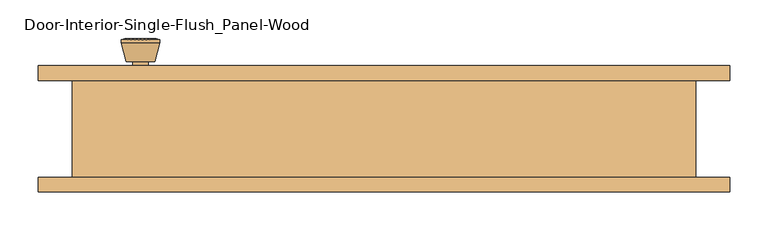
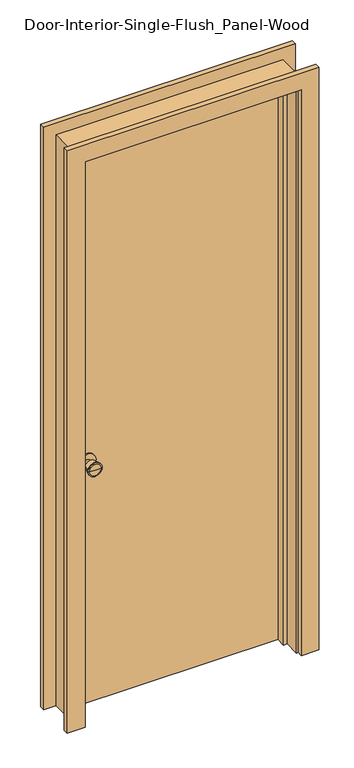
"""IFC4 building model written with IfcOpenShell, lengths in millimetres: door geometry, Door-Interior-Single-Flush_Panel-Wood."""

from ifc_helpers import new_model, si_unit, point, frame, frame_2d, origin, origin_with_axes, place, context, project, spatial, polyline, circle_curve, trimmed, segment, composite_curve, outline, extrude, faceted_brep, source, transform, mapped, element, save
from ifc_brep_helpers import plane_surface, cylinder_surface, revolved_surface, advanced_brep


def door_interior_single_flush_panel_wood_df77f4d3(model_context):
    return source(origin(), model_context, "Body", "SolidModel", [
        advanced_brep(
        [(-317.5, 19.4, 914.4), (-307.5, 19.4, 914.4), (-327.5, 19.4, 914.4), (-297.0241324, -29.6, 914.4), (-317.5, -29.6, 914.4), (-337.9758676, -29.6, 914.4), (-292.5, -27.7721319, 914.4), (-342.5, -27.7721319, 914.4), (-292.5, -24.3084537, 914.4), (-342.5, -24.3084537, 914.4), (-298.863764, 0.4, 914.4), (-336.136236, 0.4, 914.4), (-307.5, 0.4, 914.4), (-327.5, 0.4, 914.4)],
        [
            (0, 1),
            (1, 2, circle_curve(frame((-317.5, 19.4, 914.4), z_axis=(0.0, 1.0, 0.0), x_axis=(-1.0, 0.0, 0.0)), 10.0)),
            (2, 0),
            (2, 1, circle_curve(frame((-317.5, 19.4, 914.4), z_axis=(0.0, 1.0, 0.0), x_axis=(-1.0, 0.0, 0.0)), 10.0)),
            (3, 4),
            (4, 5),
            (5, 3, circle_curve(frame((-317.5, -29.6, 914.4), z_axis=(0.0, -1.0, 0.0), x_axis=(-1.0, 0.0, 0.0)), 20.4758676)),
            (3, 5, circle_curve(frame((-317.5, -29.6, 914.4), z_axis=(0.0, -1.0, 0.0), x_axis=(-1.0, 0.0, 0.0)), 20.4758676)),
            (6, 3),
            (5, 7),
            (7, 6, circle_curve(frame((-317.5, -27.7721319, 914.4), z_axis=(0.0, -1.0, 0.0), x_axis=(-1.0, 0.0, 0.0)), 25.0)),
            (6, 7, circle_curve(frame((-317.5, -27.7721319, 914.4), z_axis=(0.0, -1.0, 0.0), x_axis=(-1.0, 0.0, 0.0)), 25.0)),
            (8, 6),
            (7, 9),
            (9, 8, circle_curve(frame((-317.5, -24.3084537, 914.4), z_axis=(0.0, -1.0, 0.0), x_axis=(-1.0, 0.0, 0.0)), 25.0)),
            (8, 9, circle_curve(frame((-317.5, -24.3084537, 914.4), z_axis=(0.0, -1.0, 0.0), x_axis=(-1.0, 0.0, 0.0)), 25.0)),
            (10, 8),
            (9, 11),
            (11, 10, circle_curve(frame((-317.5, 0.4, 914.4), z_axis=(0.0, -1.0, 0.0), x_axis=(-1.0, 0.0, 0.0)), 18.636236)),
            (10, 11, circle_curve(frame((-317.5, 0.4, 914.4), z_axis=(0.0, -1.0, 0.0), x_axis=(-1.0, 0.0, 0.0)), 18.636236)),
            (12, 10),
            (11, 13),
            (13, 12, circle_curve(frame((-317.5, 0.4, 914.4), z_axis=(0.0, -1.0, 0.0), x_axis=(-1.0, 0.0, 0.0)), 10.0)),
            (12, 13, circle_curve(frame((-317.5, 0.4, 914.4), z_axis=(0.0, -1.0, 0.0), x_axis=(-1.0, 0.0, 0.0)), 10.0)),
            (1, 12),
            (13, 2),
        ],
        [
            plane_surface(frame((-317.5, 19.4, 914.4), z_axis=(0.0, 1.0, 0.0), x_axis=(-1.0, 0.0, 0.0))),
            plane_surface(frame((-317.5, -29.6, 914.4), z_axis=(0.0, -1.0, 0.0), x_axis=(-1.0, 0.0, 0.0))),
            revolved_surface(polyline([(-337.9758676, -29.6, 914.4), (-342.5, -27.7721319, 914.4)]), (-317.5, 19.4, 914.4), (0.0, 1.0, 0.0)),
            cylinder_surface(frame((-317.5, 19.4, 914.4), z_axis=(0.0, 1.0, 0.0), x_axis=(-1.0, 0.0, 0.0)), 25.0),
            revolved_surface(polyline([(-342.5, -24.3084537, 914.4), (-336.136236, 0.4, 914.4)]), (-317.5, 19.4, 914.4), (0.0, 1.0, 0.0)),
            plane_surface(frame((-317.5, 0.4, 914.4), z_axis=(0.0, 1.0, 0.0), x_axis=(-1.0, 0.0, 0.0))),
            cylinder_surface(frame((-317.5, 19.4, 914.4), z_axis=(0.0, 1.0, 0.0), x_axis=(-1.0, 0.0, 0.0)), 10.0),
        ],
        [
            (0, [[1, 2, 3]]),
            (0, [[-3, 4, -1]]),
            (1, [[5, 6, 7]]),
            (1, [[-6, -5, 8]]),
            (2, [[9, -7, 10, 11]]),
            (2, [[-10, -8, -9, 12]]),
            (3, [[13, -11, 14, 15]]),
            (3, [[-14, -12, -13, 16]]),
            (4, [[17, -15, 18, 19]]),
            (4, [[-18, -16, -17, 20]]),
            (5, [[21, -19, 22, 23]]),
            (5, [[-22, -20, -21, 24]]),
            (6, [[25, -23, 26, -2]]),
            (6, [[-26, -24, -25, -4]]),
        ],
    ),
        extrude(outline(composite_curve([segment(trimmed(circle_curve(frame_2d((914.4, -317.5)), 30.0), [point((914.4, -347.5))], [point((914.4, -287.5))], False, "CARTESIAN"), True, "CONTINUOUS"), segment(trimmed(circle_curve(frame_2d((914.4, -317.5)), 30.0), [point((914.4, -287.5))], [point((914.4, -347.5))], False, "CARTESIAN"), True, "CONTINUOUS")], self_intersect=False)), frame((0.0, 19.4, 0.0), z_axis=(0.0, 1.0, 0.0), x_axis=(0.0, 0.0, 1.0)), (0.0, 0.0, 1.0), 6.0),
        advanced_brep(
        [(-317.5, 66.325, 914.4), (-327.5, 66.325, 914.4), (-307.5, 66.325, 914.4), (-297.0241324, 115.325, 914.4), (-337.9758676, 115.325, 914.4), (-317.5, 115.325, 914.4), (-292.5, 113.4971319, 914.4), (-342.5, 113.4971319, 914.4), (-292.5, 110.0334537, 914.4), (-342.5, 110.0334537, 914.4), (-298.863764, 85.325, 914.4), (-336.136236, 85.325, 914.4), (-307.5, 85.325, 914.4), (-327.5, 85.325, 914.4)],
        [
            (0, 1),
            (1, 2, circle_curve(frame((-317.5, 66.325, 914.4), z_axis=(0.0, -1.0, 0.0), x_axis=(-1.0, 0.0, 0.0)), 10.0)),
            (2, 0),
            (2, 1, circle_curve(frame((-317.5, 66.325, 914.4), z_axis=(0.0, -1.0, 0.0), x_axis=(-1.0, 0.0, 0.0)), 10.0)),
            (3, 4, circle_curve(frame((-317.5, 115.325, 914.4), z_axis=(0.0, 1.0, 0.0), x_axis=(-1.0, 0.0, 0.0)), 20.4758676)),
            (4, 5),
            (5, 3),
            (4, 3, circle_curve(frame((-317.5, 115.325, 914.4), z_axis=(0.0, 1.0, 0.0), x_axis=(-1.0, 0.0, 0.0)), 20.4758676)),
            (6, 7, circle_curve(frame((-317.5, 113.4971319, 914.4), z_axis=(0.0, 1.0, 0.0), x_axis=(-1.0, 0.0, 0.0)), 25.0)),
            (7, 4),
            (3, 6),
            (7, 6, circle_curve(frame((-317.5, 113.4971319, 914.4), z_axis=(0.0, 1.0, 0.0), x_axis=(-1.0, 0.0, 0.0)), 25.0)),
            (8, 9, circle_curve(frame((-317.5, 110.0334537, 914.4), z_axis=(0.0, 1.0, 0.0), x_axis=(-1.0, 0.0, 0.0)), 25.0)),
            (9, 7),
            (6, 8),
            (9, 8, circle_curve(frame((-317.5, 110.0334537, 914.4), z_axis=(0.0, 1.0, 0.0), x_axis=(-1.0, 0.0, 0.0)), 25.0)),
            (10, 11, circle_curve(frame((-317.5, 85.325, 914.4), z_axis=(0.0, 1.0, 0.0), x_axis=(-1.0, 0.0, 0.0)), 18.636236)),
            (11, 9),
            (8, 10),
            (11, 10, circle_curve(frame((-317.5, 85.325, 914.4), z_axis=(0.0, 1.0, 0.0), x_axis=(-1.0, 0.0, 0.0)), 18.636236)),
            (12, 13, circle_curve(frame((-317.5, 85.325, 914.4), z_axis=(0.0, 1.0, 0.0), x_axis=(-1.0, 0.0, 0.0)), 10.0)),
            (13, 11),
            (10, 12),
            (13, 12, circle_curve(frame((-317.5, 85.325, 914.4), z_axis=(0.0, 1.0, 0.0), x_axis=(-1.0, 0.0, 0.0)), 10.0)),
            (1, 13),
            (12, 2),
        ],
        [
            plane_surface(frame((-317.5, 66.325, 914.4), z_axis=(0.0, -1.0, 0.0), x_axis=(-1.0, 0.0, 0.0))),
            plane_surface(frame((-317.5, 115.325, 914.4), z_axis=(0.0, 1.0, 0.0), x_axis=(-1.0, 0.0, 0.0))),
            revolved_surface(polyline([(-337.9758676, 115.325, 914.4), (-342.5, 113.4971319, 914.4)]), (-317.5, 66.325, 914.4), (0.0, -1.0, 0.0)),
            cylinder_surface(frame((-317.5, 66.325, 914.4), z_axis=(0.0, -1.0, 0.0), x_axis=(-1.0, 0.0, 0.0)), 25.0),
            revolved_surface(polyline([(-342.5, 110.0334537, 914.4), (-336.136236, 85.325, 914.4)]), (-317.5, 66.325, 914.4), (0.0, -1.0, 0.0)),
            plane_surface(frame((-317.5, 85.325, 914.4), z_axis=(0.0, -1.0, 0.0), x_axis=(-1.0, 0.0, 0.0))),
            cylinder_surface(frame((-317.5, 66.325, 914.4), z_axis=(0.0, -1.0, 0.0), x_axis=(-1.0, 0.0, 0.0)), 10.0),
        ],
        [
            (0, [[1, 2, 3]]),
            (0, [[-3, 4, -1]]),
            (1, [[5, 6, 7]]),
            (1, [[8, -7, -6]]),
            (2, [[9, 10, -5, 11]]),
            (2, [[12, -11, -8, -10]]),
            (3, [[13, 14, -9, 15]]),
            (3, [[16, -15, -12, -14]]),
            (4, [[17, 18, -13, 19]]),
            (4, [[20, -19, -16, -18]]),
            (5, [[21, 22, -17, 23]]),
            (5, [[24, -23, -20, -22]]),
            (6, [[-2, 25, -21, 26]]),
            (6, [[-4, -26, -24, -25]]),
        ],
    ),
        extrude(outline(composite_curve([segment(trimmed(circle_curve(frame_2d((914.4, -317.5)), 30.0), [point((914.4, -347.5))], [point((914.4, -287.5))], False, "CARTESIAN"), True, "CONTINUOUS"), segment(trimmed(circle_curve(frame_2d((914.4, -317.5)), 30.0), [point((914.4, -287.5))], [point((914.4, -347.5))], False, "CARTESIAN"), True, "CONTINUOUS")], self_intersect=False)), frame((0.0, 60.325, 0.0), z_axis=(0.0, 1.0, 0.0), x_axis=(0.0, 0.0, 1.0)), (0.0, 0.0, 1.0), 6.0),
        extrude(outline(polyline([(381.0, 25.4), (-381.0, 25.4), (-381.0, 60.325), (381.0, 60.325), (381.0, 25.4)])), origin_with_axes(), (0.0, 0.0, 1.0), 2133.6),
        faceted_brep([(406.4, 60.325, 0.0), (406.4, -66.675, 0.0), (381.0, -66.675, 0.0), (381.0, -9.525, 0.0), (368.3, -9.525, 0.0), (368.3, 25.4, 0.0), (381.0, 25.4, 0.0), (381.0, 60.325, 0.0), (406.4, 60.325, 2159.0), (406.4, -66.675, 2159.0), (-406.4, -66.675, 2159.0), (-406.4, -66.675, 0.0), (-381.0, -66.675, 0.0), (-381.0, -66.675, 2133.6), (381.0, -66.675, 2133.6), (381.0, -9.525, 2133.6), (-381.0, -9.525, 2133.6), (-381.0, -9.525, 0.0), (-368.3, -9.525, 0.0), (-368.3, -9.525, 2120.9), (368.3, -9.525, 2120.9), (368.3, 25.4, 2120.9), (-368.3, 25.4, 2120.9), (-368.3, 25.4, 0.0), (-381.0, 25.4, 0.0), (-381.0, 25.4, 2133.6), (381.0, 25.4, 2133.6), (381.0, 60.325, 2133.6), (-381.0, 60.325, 2133.6), (-381.0, 60.325, 0.0), (-406.4, 60.325, 0.0), (-406.4, 60.325, 2159.0)], [[[0, 1, 2, 3, 4, 5, 6, 7]], [[1, 0, 8, 9]], [[2, 1, 9, 10, 11, 12, 13, 14]], [[3, 2, 14, 15]], [[4, 3, 15, 16, 17, 18, 19, 20]], [[5, 4, 20, 21]], [[6, 5, 21, 22, 23, 24, 25, 26]], [[7, 6, 26, 27]], [[0, 7, 27, 28, 29, 30, 31, 8]], [[9, 8, 31, 10]], [[15, 14, 13, 16]], [[21, 20, 19, 22]], [[27, 26, 25, 28]], [[30, 29, 24, 23, 18, 17, 12, 11]], [[10, 31, 30, 11]], [[16, 13, 12, 17]], [[22, 19, 18, 23]], [[28, 25, 24, 29]]]),
        extrude(outline(polyline([(0.0, 387.35), (0.0, 450.85), (2203.45, 450.85), (2203.45, -450.85), (0.0, -450.85), (0.0, -387.35), (2139.95, -387.35), (2139.95, 387.35), (0.0, 387.35)])), frame((0.0, -85.725, 0.0), z_axis=(0.0, 1.0, 0.0), x_axis=(0.0, 0.0, 1.0)), (0.0, 0.0, 1.0), 19.05),
        extrude(outline(polyline([(0.0, 387.35), (0.0, 450.85), (2203.45, 450.85), (2203.45, -450.85), (0.0, -450.85), (0.0, -387.35), (2139.95, -387.35), (2139.95, 387.35), (0.0, 387.35)])), frame((0.0, 60.325, 0.0), z_axis=(0.0, 1.0, 0.0), x_axis=(0.0, 0.0, 1.0)), (0.0, 0.0, 1.0), 19.05),
    ])


if __name__ == "__main__":
    model = new_model("IFC4")
    model_context = context("Model", 3, world=origin())
    ifc_project = project(units=[si_unit("LENGTHUNIT", "METRE", prefix="MILLI")], contexts=[model_context])
    site = spatial("IfcSite", under=ifc_project)
    building = spatial("IfcBuilding", under=site)
    placement = place(None, origin())
    door_interior_single_flush_panel_wood_shape = door_interior_single_flush_panel_wood_df77f4d3(model_context)
    element("IfcDoor", 1, ObjectType="Door-Interior-Single-Flush_Panel-Wood", at=placement, inside=building, context=model_context, shape_type="MappedRepresentation", body=[
        mapped(door_interior_single_flush_panel_wood_shape, transform((0.0, 0.0, 0.0), x_axis=(1.0, 0.0, 0.0), y_axis=(0.0, 1.0, 0.0), z_axis=(0.0, 0.0, 1.0))),
    ])
    save(model, "model.ifc")

# Revit data of these elements
# Type "Door-Interior-Single-Flush_Panel-Wood"
#   Type Mark = "13"
#   Assembly Code = "C1020300"
#   Analytic Construction = "Wooden"
#   Thickness = 0' - 1 3/8"
#   Thermal Resistance (R) = 2.5876 (h·ft²·°F)/BTU
#   Swing Angle [instance default] = 90.00°
#   Rough Width = 2' - 8"
#   Rough Height = 7' - 1"
#   Height = 7' - 0"
#   Width = 2' - 6"
#   Heat Transfer Coefficient (U) = 0.3865 BTU/(h·ft²·°F)
#   Trim Material = Cherry
#   Panel Material = Cherry
#   Frame Material = Cherry
#   Door Handle Material = Aluminum
#   Visual Light Transmittance = 0
#   Solar Heat Gain Coefficient = 0
#   Wall Closure = (empty or 0)
#   Function = (empty or 0)
# Element 1 (IfcDoor, "Door-Interior-Single-Flush_Panel-Wood")
#   Materials on its faces: "Cherry", "Aluminum"
# Materials
#   "Cherry": class "Wood", colour RGB 226 177 128, transparency 0, Description = "Prunus Serotina", Cost = 0
#   "Aluminum": class "Metal", colour RGB 247 247 247, transparency 0, Description = "Aluminum 6061", Cost = 0
